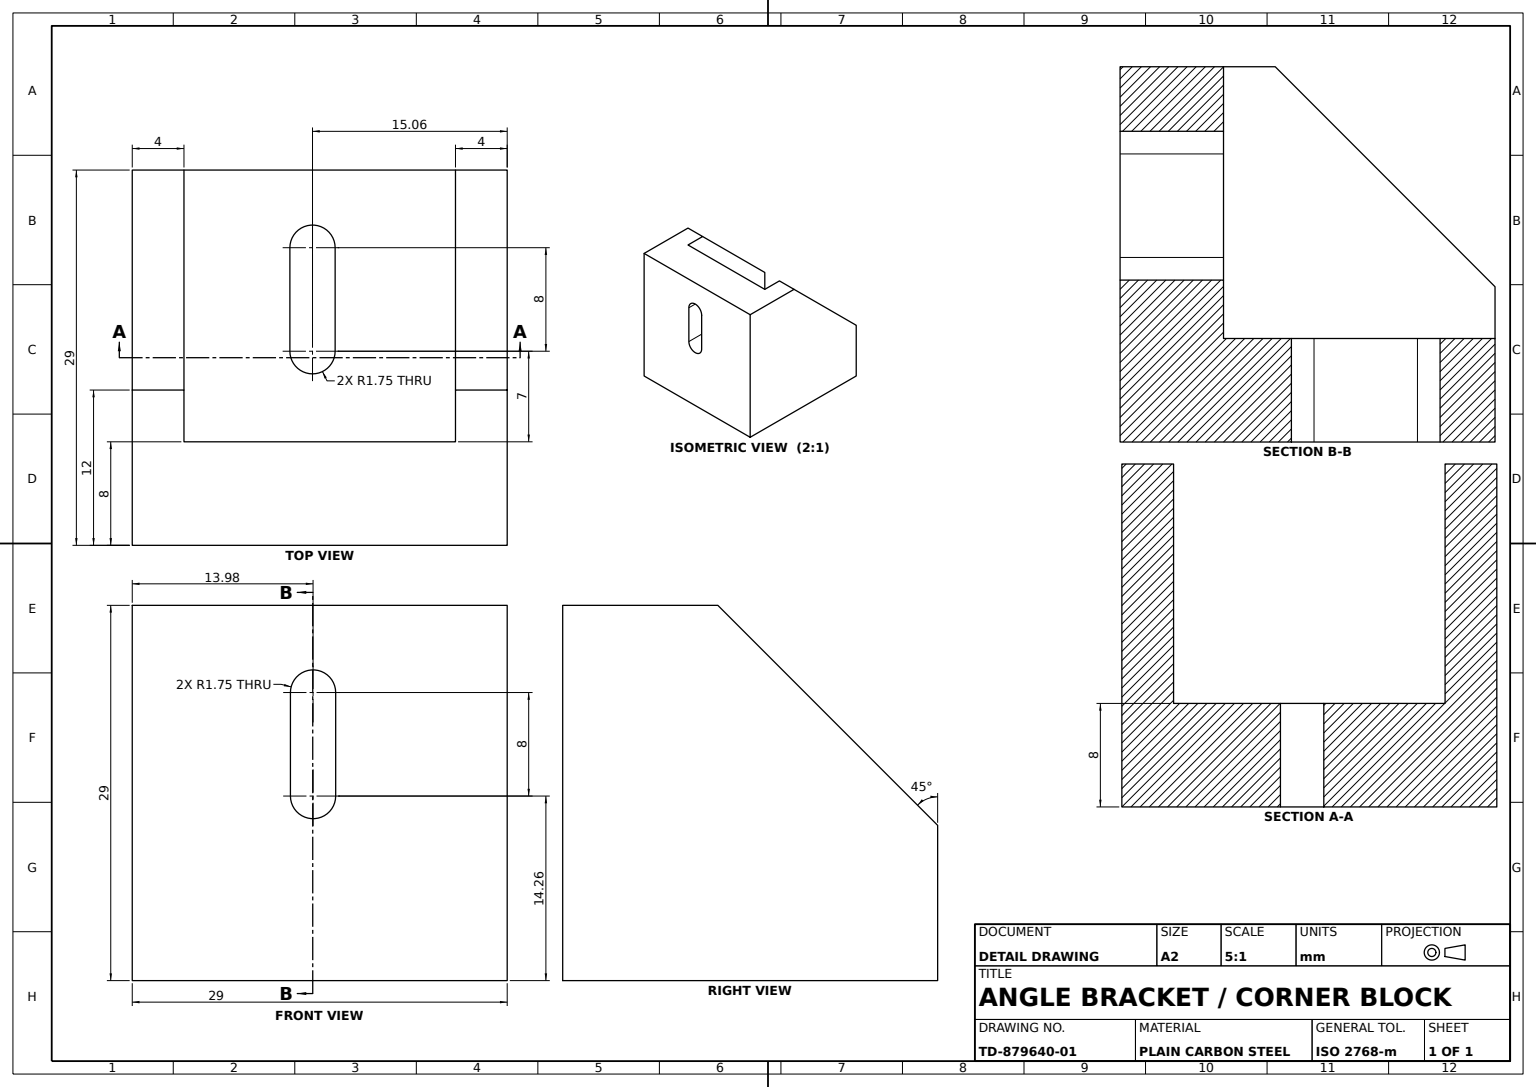
from build123d import *

# Parameters (mm, degrees)
BASE_PLATE_SKETCH_W    = 29
BASE_PLATE_SKETCH_H    = 29
BASE_PLATE_8MM_DEPTH   = 8
BASE_SLOT_3_5MM_DEPTH  = 8
UPRIGHT_WALL_SKETCH_W  = 29
UPRIGHT_WALL_SKETCH_H  = 21
UPRIGHT_WALL_8MM_DEPTH = 8
WALL_SLOT_3_5MM_DEPTH  = 8
SIDE_BOSS_A_4MM_DEPTH  = 4
SIDE_BOSS_B_4MM_DEPTH  = 4


with BuildPart() as part:
    # Base Plate Sketch → Base Plate 8mm (new body)
    with BuildSketch(Plane.XY):
        with Locations((14.5, 14.5)):
            Rectangle(BASE_PLATE_SKETCH_W, BASE_PLATE_SKETCH_H)
    extrude(amount=BASE_PLATE_8MM_DEPTH)

    # Base Slot Sketch → Base Slot 3.5mm (cut)
    with BuildSketch(Plane.XY.offset(8)):
        with BuildLine():
            Line((12.234144505, 22.262653084), (12.234144505, 14.262653084))
            ThreePointArc((12.234144505, 14.262653084), (13.984144505, 12.512653084), (15.734144505, 14.262653084))
            Line((15.734144505, 14.262653084), (15.734144505, 22.262653084))
            ThreePointArc((15.734144505, 22.262653084), (13.984144505, 24.012653084), (12.234144505, 22.262653084))
        make_face()
    extrude(amount=-BASE_SLOT_3_5MM_DEPTH, mode=Mode.SUBTRACT)

    # Upright Wall Sketch → Upright Wall 8mm (add)
    with BuildSketch(Plane.XZ):
        with Locations((14.5, -10.5)):
            Rectangle(UPRIGHT_WALL_SKETCH_W, UPRIGHT_WALL_SKETCH_H)
    extrude(amount=-UPRIGHT_WALL_8MM_DEPTH)

    # Wall Slot Sketch → Wall Slot 3.5mm (cut)
    with BuildSketch(Plane(origin=(0, 8, 0), x_dir=(1, 0, 0), z_dir=(0, 1, 0))):
        with BuildLine():
            Line((12.192184218, 15), (12.192184218, 7))
            ThreePointArc((12.192184218, 7), (13.942184218, 5.25), (15.692184218, 7))
            Line((15.692184218, 7), (15.692184218, 15))
            ThreePointArc((15.692184218, 15), (13.942184218, 16.75), (12.192184218, 15))
        make_face()
    extrude(amount=-WALL_SLOT_3_5MM_DEPTH, mode=Mode.SUBTRACT)

    # Side Boss A Sketch → Side Boss A 4mm (add)
    with BuildSketch(Plane(origin=(29, 0, 0), x_dir=(0, 0, -1), z_dir=(1, 0, 0))):
        Polygon((0, 29), (4, 29), (21, 12), (21, 8), (0, 8), align=None)
    extrude(amount=-SIDE_BOSS_A_4MM_DEPTH)

    # Side Boss B Sketch → Side Boss B 4mm (add)
    with BuildSketch(Plane.ZY):
        Polygon((0, 29), (-4, 29), (-21, 12), (-21, 8), (0, 8), align=None)
    extrude(amount=-SIDE_BOSS_B_4MM_DEPTH)


solid = part.part
